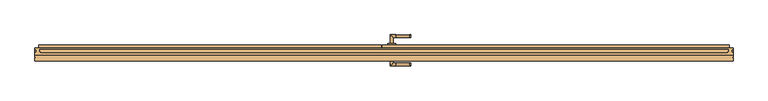
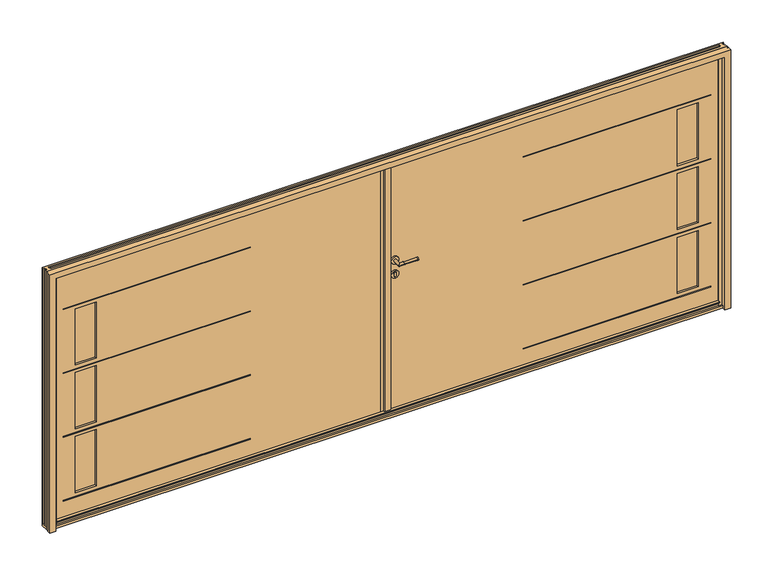
"""IFC4 building model written with IfcOpenShell, lengths in millimetres: door geometry."""

from ifc_helpers import new_model, si_unit, point, frame, frame_2d, origin, origin_with_axes, place, context, project, spatial, polyline, circle_curve, ellipse_curve, trimmed, segment, composite_curve, outline, extrude, faceted_brep, source, transform, mapped, element, save
from ifc_brep_helpers import plane_surface, cylinder_surface, advanced_brep


def door_2a186d26(model_context):
    return source(origin(), model_context, "Body", "SolidModel", [
        extrude(outline(polyline([(2198.0, 21.5), (82.0, 21.5), (82.0, 49.5), (2198.0, 49.5), (2198.0, 21.5)])), frame((0.0, 0.0, 108.0), z_axis=(0.0, 0.0, 1.0), x_axis=(1.0, 0.0, 0.0)), (0.0, 0.0, 1.0), 1633.8),
        advanced_brep(
        [(60.1308541, 82.5, 1120.0), (41.1308541, 82.5, 1120.0), (60.1308541, 123.5, 1120.0), (41.1308541, 142.5, 1120.0), (176.1308541, 123.5, 1120.0), (176.1308541, 142.5, 1120.0), (79.1308541, 123.5, 1120.0), (79.1308541, 142.5, 1120.0), (170.1308541, 142.5, 1120.0), (170.1308541, 123.5, 1120.0), (170.1308541, 124.0, 1120.0), (170.1308541, 142.0, 1120.0), (79.1308541, 124.0, 1120.0), (79.1308541, 142.0, 1120.0)],
        [
            (0, 1, circle_curve(frame((50.6308541, 82.5, 1120.0), z_axis=(0.0, -1.0, 0.0), x_axis=(-1.0, 0.0, 0.0)), 9.5)),
            (1, 0, circle_curve(frame((50.6308541, 82.5, 1120.0), z_axis=(0.0, -1.0, 0.0), x_axis=(-1.0, 0.0, 0.0)), 9.5)),
            (0, 2),
            (2, 3, ellipse_curve(frame((50.6308541, 133.0, 1120.0), z_axis=(-0.7071067811865475, -0.7071067811865475, 0.0), x_axis=(0.7071067811865474, -0.7071067811865476, 0.0)), 13.4350288, 9.5)),
            (3, 1),
            (3, 2, ellipse_curve(frame((50.6308541, 133.0, 1120.0), z_axis=(-0.7071067811865475, -0.7071067811865475, 0.0), x_axis=(0.7071067811865474, -0.7071067811865476, 0.0)), 13.4350288, 9.5)),
            (4, 5, circle_curve(frame((176.1308541, 133.0, 1120.0), z_axis=(1.0, 0.0, 0.0), x_axis=(0.0, 1.0, 0.0)), 9.5)),
            (5, 4, circle_curve(frame((176.1308541, 133.0, 1120.0), z_axis=(1.0, 0.0, 0.0), x_axis=(0.0, 1.0, 0.0)), 9.5)),
            (2, 6),
            (6, 7, circle_curve(frame((79.1308541, 133.0, 1120.0), z_axis=(-1.0, 0.0, 0.0), x_axis=(0.0, 1.0, 0.0)), 9.5)),
            (7, 3),
            (5, 8),
            (8, 9, circle_curve(frame((170.1308541, 133.0, 1120.0), z_axis=(1.0, 0.0, 0.0), x_axis=(0.0, 1.0, 0.0)), 9.5)),
            (9, 4),
            (7, 6, circle_curve(frame((79.1308541, 133.0, 1120.0), z_axis=(-1.0, 0.0, 0.0), x_axis=(0.0, 1.0, 0.0)), 9.5)),
            (9, 8, circle_curve(frame((170.1308541, 133.0, 1120.0), z_axis=(1.0, 0.0, 0.0), x_axis=(0.0, 1.0, 0.0)), 9.5)),
            (10, 11, circle_curve(frame((170.1308541, 133.0, 1120.0), z_axis=(1.0, 0.0, 0.0), x_axis=(0.0, 1.0, 0.0)), 9.0)),
            (11, 10, circle_curve(frame((170.1308541, 133.0, 1120.0), z_axis=(1.0, 0.0, 0.0), x_axis=(0.0, 1.0, 0.0)), 9.0)),
            (12, 13, circle_curve(frame((79.1308541, 133.0, 1120.0), z_axis=(-1.0, 0.0, 0.0), x_axis=(0.0, 1.0, 0.0)), 9.0)),
            (13, 12, circle_curve(frame((79.1308541, 133.0, 1120.0), z_axis=(-1.0, 0.0, 0.0), x_axis=(0.0, 1.0, 0.0)), 9.0)),
            (11, 13),
            (12, 10),
        ],
        [
            plane_surface(frame((50.6308541, 82.5, 1120.0), z_axis=(0.0, -1.0, 0.0), x_axis=(0.0, 0.0, 1.0))),
            cylinder_surface(frame((50.6308541, 82.5, 1120.0), z_axis=(0.0, -1.0, 0.0), x_axis=(-1.0, 0.0, 0.0)), 9.5),
            plane_surface(frame((176.1308541, 133.0, 1120.0), z_axis=(1.0, 0.0, 0.0), x_axis=(0.0, 0.0, 1.0))),
            cylinder_surface(frame((50.6308541, 133.0, 1120.0), z_axis=(-1.0, 0.0, 0.0), x_axis=(0.0, 1.0, 0.0)), 9.5),
            plane_surface(frame((170.1308541, 142.5, 1120.0), z_axis=(-1.0, 0.0, 0.0), x_axis=(0.0, 0.0, 1.0))),
            plane_surface(frame((79.1308541, 142.5, 1120.0), z_axis=(1.0, 0.0, 0.0), x_axis=(0.0, 0.0, -1.0))),
            cylinder_surface(frame((50.6308541, 133.0, 1120.0), z_axis=(-1.0, 0.0, 0.0), x_axis=(0.0, 1.0, 0.0)), 9.0),
        ],
        [
            (0, [[1, 2]]),
            (1, [[-1, 3, 4, 5]]),
            (1, [[-2, -5, 6, -3]]),
            (2, [[7, 8]]),
            (3, [[-4, 9, 10, 11]]),
            (3, [[-8, 12, 13, 14]]),
            (3, [[-6, -11, 15, -9]]),
            (3, [[-7, -14, 16, -12]]),
            (4, [[-13, -16], [17, 18]]),
            (5, [[-10, -15], [19, 20]]),
            (6, [[-18, 21, -19, 22]]),
            (6, [[-17, -22, -20, -21]]),
        ],
    ),
        extrude(outline(composite_curve([segment(trimmed(circle_curve(frame_2d((1019.75, 50.6308541)), 26.0), [point((1019.75, 24.6308541))], [point((1019.75, 76.6308541))], False, "CARTESIAN"), True, "CONTINUOUS"), segment(trimmed(circle_curve(frame_2d((1019.75, 50.6308541)), 26.0), [point((1019.75, 76.6308541))], [point((1019.75, 24.6308541))], False, "CARTESIAN"), True, "CONTINUOUS")], self_intersect=False)), frame((0.0, 72.5, 0.0), z_axis=(0.0, 1.0, 0.0), x_axis=(0.0, 0.0, 1.0)), (0.0, 0.0, 1.0), 10.0),
        extrude(outline(composite_curve([segment(polyline([(1021.404547, 44.8808541), (1008.0, 44.8808541)]), True, "CONTINUOUS"), segment(trimmed(circle_curve(frame_2d((1008.0, 50.6308541)), 5.75), [point((1008.0, 44.8808541))], [point((1008.0, 56.3808541))], False, "CARTESIAN"), True, "CONTINUOUS"), segment(polyline([(1008.0, 56.3808541), (1021.404547, 56.3808541)]), True, "CONTINUOUS"), segment(trimmed(circle_curve(frame_2d((1028.0, 50.6308541)), 8.75), [point((1021.404547, 56.3808541))], [point((1021.404547, 44.8808541))], False, "CARTESIAN"), True, "CONTINUOUS")], self_intersect=False)), frame((0.0, 82.5, 0.0), z_axis=(0.0, 1.0, 0.0), x_axis=(0.0, 0.0, 1.0)), (0.0, 0.0, 1.0), 1.0),
        extrude(outline(composite_curve([segment(trimmed(circle_curve(frame_2d((1120.0, 50.6308541)), 26.0), [point((1120.0, 24.6308541))], [point((1120.0, 76.6308541))], False, "CARTESIAN"), True, "CONTINUOUS"), segment(trimmed(circle_curve(frame_2d((1120.0, 50.6308541)), 26.0), [point((1120.0, 76.6308541))], [point((1120.0, 24.6308541))], False, "CARTESIAN"), True, "CONTINUOUS")], self_intersect=False)), frame((0.0, 72.5, 0.0), z_axis=(0.0, 1.0, 0.0), x_axis=(0.0, 0.0, 1.0)), (0.0, 0.0, 1.0), 10.0),
        advanced_brep(
        [(60.1308541, -4.5, 1120.0), (41.1308541, -4.5, 1120.0), (41.1308541, -64.5, 1120.0), (60.1308541, -45.5, 1120.0), (176.1308541, -45.5, 1120.0), (176.1308541, -64.5, 1120.0), (170.1308541, -45.5, 1120.0), (170.1308541, -64.5, 1120.0), (79.1308541, -64.5, 1120.0), (79.1308541, -45.5, 1120.0), (170.1308541, -46.0, 1120.0), (170.1308541, -64.0, 1120.0), (79.1308541, -46.0, 1120.0), (79.1308541, -64.0, 1120.0)],
        [
            (0, 1, circle_curve(frame((50.6308541, -4.5, 1120.0), z_axis=(0.0, 1.0, 0.0), x_axis=(-1.0, 0.0, 0.0)), 9.5)),
            (1, 0, circle_curve(frame((50.6308541, -4.5, 1120.0), z_axis=(0.0, 1.0, 0.0), x_axis=(-1.0, 0.0, 0.0)), 9.5)),
            (1, 2),
            (2, 3, ellipse_curve(frame((50.6308541, -55.0, 1120.0), z_axis=(-0.7071067811865475, 0.7071067811865475, 0.0), x_axis=(0.7071067811865474, 0.7071067811865476, 0.0)), 13.4350288, 9.5)),
            (3, 0),
            (3, 2, ellipse_curve(frame((50.6308541, -55.0, 1120.0), z_axis=(-0.7071067811865475, 0.7071067811865475, 0.0), x_axis=(0.7071067811865474, 0.7071067811865476, 0.0)), 13.4350288, 9.5)),
            (4, 5, circle_curve(frame((176.1308541, -55.0, 1120.0), z_axis=(1.0, 0.0, 0.0), x_axis=(0.0, -1.0, 0.0)), 9.5)),
            (5, 4, circle_curve(frame((176.1308541, -55.0, 1120.0), z_axis=(1.0, 0.0, 0.0), x_axis=(0.0, -1.0, 0.0)), 9.5)),
            (4, 6),
            (6, 7, circle_curve(frame((170.1308541, -55.0, 1120.0), z_axis=(1.0, 0.0, 0.0), x_axis=(0.0, -1.0, 0.0)), 9.5)),
            (7, 5),
            (2, 8),
            (8, 9, circle_curve(frame((79.1308541, -55.0, 1120.0), z_axis=(-1.0, 0.0, 0.0), x_axis=(0.0, -1.0, 0.0)), 9.5)),
            (9, 3),
            (9, 8, circle_curve(frame((79.1308541, -55.0, 1120.0), z_axis=(-1.0, 0.0, 0.0), x_axis=(0.0, -1.0, 0.0)), 9.5)),
            (7, 6, circle_curve(frame((170.1308541, -55.0, 1120.0), z_axis=(1.0, 0.0, 0.0), x_axis=(0.0, -1.0, 0.0)), 9.5)),
            (10, 11, circle_curve(frame((170.1308541, -55.0, 1120.0), z_axis=(1.0, 0.0, 0.0), x_axis=(0.0, -1.0, 0.0)), 9.0)),
            (11, 10, circle_curve(frame((170.1308541, -55.0, 1120.0), z_axis=(1.0, 0.0, 0.0), x_axis=(0.0, -1.0, 0.0)), 9.0)),
            (12, 13, circle_curve(frame((79.1308541, -55.0, 1120.0), z_axis=(-1.0, 0.0, 0.0), x_axis=(0.0, -1.0, 0.0)), 9.0)),
            (13, 12, circle_curve(frame((79.1308541, -55.0, 1120.0), z_axis=(-1.0, 0.0, 0.0), x_axis=(0.0, -1.0, 0.0)), 9.0)),
            (10, 12),
            (13, 11),
        ],
        [
            plane_surface(frame((50.6308541, -4.5, 1120.0), z_axis=(0.0, 1.0, 0.0), x_axis=(0.0, 0.0, 1.0))),
            cylinder_surface(frame((50.6308541, -4.5, 1120.0), z_axis=(0.0, 1.0, 0.0), x_axis=(-1.0, 0.0, 0.0)), 9.5),
            plane_surface(frame((176.1308541, -55.0, 1120.0), z_axis=(1.0, 0.0, 0.0), x_axis=(0.0, 0.0, 1.0))),
            cylinder_surface(frame((50.6308541, -55.0, 1120.0), z_axis=(-1.0, 0.0, 0.0), x_axis=(0.0, -1.0, 0.0)), 9.5),
            plane_surface(frame((170.1308541, -64.5, 1120.0), z_axis=(-1.0, 0.0, 0.0), x_axis=(0.0, 0.0, 1.0))),
            plane_surface(frame((79.1308541, -64.5, 1120.0), z_axis=(1.0, 0.0, 0.0), x_axis=(0.0, 0.0, -1.0))),
            cylinder_surface(frame((50.6308541, -55.0, 1120.0), z_axis=(-1.0, 0.0, 0.0), x_axis=(0.0, -1.0, 0.0)), 9.0),
        ],
        [
            (0, [[1, 2]]),
            (1, [[3, 4, 5, -2]]),
            (1, [[-5, 6, -3, -1]]),
            (2, [[7, 8]]),
            (3, [[9, 10, 11, -7]]),
            (3, [[12, 13, 14, -4]]),
            (3, [[-14, 15, -12, -6]]),
            (3, [[-11, 16, -9, -8]]),
            (4, [[-16, -10], [17, 18]]),
            (5, [[-15, -13], [19, 20]]),
            (6, [[21, -20, 22, -17]]),
            (6, [[-22, -19, -21, -18]]),
        ],
    ),
        extrude(outline(composite_curve([segment(trimmed(circle_curve(frame_2d((1019.75, 50.6308541)), 26.0), [point((1019.75, 24.6308541))], [point((1019.75, 76.6308541))], False, "CARTESIAN"), True, "CONTINUOUS"), segment(trimmed(circle_curve(frame_2d((1019.75, 50.6308541)), 26.0), [point((1019.75, 76.6308541))], [point((1019.75, 24.6308541))], False, "CARTESIAN"), True, "CONTINUOUS")], self_intersect=False)), frame((0.0, -4.5, 0.0), z_axis=(0.0, 1.0, 0.0), x_axis=(0.0, 0.0, 1.0)), (0.0, 0.0, 1.0), 10.0),
        extrude(outline(composite_curve([segment(polyline([(1021.404547, 44.8808541), (1008.0, 44.8808541)]), True, "CONTINUOUS"), segment(trimmed(circle_curve(frame_2d((1008.0, 50.6308541)), 5.75), [point((1008.0, 44.8808541))], [point((1008.0, 56.3808541))], False, "CARTESIAN"), True, "CONTINUOUS"), segment(polyline([(1008.0, 56.3808541), (1021.404547, 56.3808541)]), True, "CONTINUOUS"), segment(trimmed(circle_curve(frame_2d((1028.0, 50.6308541)), 8.75), [point((1021.404547, 56.3808541))], [point((1021.404547, 44.8808541))], False, "CARTESIAN"), True, "CONTINUOUS")], self_intersect=False)), frame((0.0, -5.5, 0.0), z_axis=(0.0, 1.0, 0.0), x_axis=(0.0, 0.0, 1.0)), (0.0, 0.0, 1.0), 1.0),
        extrude(outline(composite_curve([segment(trimmed(circle_curve(frame_2d((1120.0, 50.6308541)), 26.0), [point((1120.0, 24.6308541))], [point((1120.0, 76.6308541))], False, "CARTESIAN"), True, "CONTINUOUS"), segment(trimmed(circle_curve(frame_2d((1120.0, 50.6308541)), 26.0), [point((1120.0, 76.6308541))], [point((1120.0, 24.6308541))], False, "CARTESIAN"), True, "CONTINUOUS")], self_intersect=False)), frame((0.0, -4.5, 0.0), z_axis=(0.0, 1.0, 0.0), x_axis=(0.0, 0.0, 1.0)), (0.0, 0.0, 1.0), 10.0),
        faceted_brep([(2262.0, 5.5, 1805.8), (2262.0, 5.5, 44.0), (2262.0, 21.4981764, 44.0), (2262.0, 21.4981764, 1805.8), (18.0, 21.5, 44.0), (18.0, 21.5, 1805.8), (1979.0, 21.5, 659.6), (2123.0, 21.5, 659.6), (2123.0, 21.5, 1065.7), (1979.0, 21.5, 1065.7), (1979.0, 21.5, 199.0), (2123.0, 21.5, 199.0), (2123.0, 21.5, 605.1), (1979.0, 21.5, 605.1), (1979.0, 21.5, 1120.2), (2123.0, 21.5, 1120.2), (2123.0, 21.5, 1526.3), (1979.0, 21.5, 1526.3), (18.0, 5.5, 44.0), (18.0, 5.5, 1805.8), (1979.0, 5.5, 1065.7), (1979.0, 5.5, 659.6), (2123.0, 5.5, 1065.7), (2123.0, 5.5, 659.6), (1979.0, 5.5, 605.1), (1979.0, 5.5, 199.0), (2123.0, 5.5, 605.1), (2123.0, 5.5, 199.0), (930.0, 5.5, 1094.2), (2206.0, 5.5, 1094.2), (2206.0, 5.5, 1089.2), (930.0, 5.5, 1089.2), (930.0, 5.5, 633.6), (2206.0, 5.5, 633.6), (2206.0, 5.5, 628.6), (930.0, 5.5, 628.6), (930.0, 5.5, 173.0), (2206.0, 5.5, 173.0), (2206.0, 5.5, 168.0), (930.0, 5.5, 168.0), (1979.0, 5.5, 1526.3), (2123.0, 5.5, 1526.3), (2123.0, 5.5, 1120.2), (1979.0, 5.5, 1120.2), (930.0, 5.5, 1554.8), (2206.0, 5.5, 1554.8), (2206.0, 5.5, 1549.8), (930.0, 5.5, 1549.8), (930.0, 14.5185028, 1094.2), (930.0, 14.5185028, 1089.2), (2206.0, 14.5185028, 1089.2), (2206.0, 14.5185028, 1094.2), (930.0, 14.5185028, 633.6), (930.0, 14.5185028, 628.6), (2206.0, 14.5185028, 628.6), (2206.0, 14.5185028, 633.6), (930.0, 14.5185028, 173.0), (930.0, 14.5185028, 168.0), (2206.0, 14.5185028, 168.0), (2206.0, 14.5185028, 173.0), (930.0, 14.5185028, 1554.8), (930.0, 14.5185028, 1549.8), (2206.0, 14.5185028, 1549.8), (2206.0, 14.5185028, 1554.8)], [[[0, 1, 2, 3]], [[2, 4, 5, 3], [6, 7, 8, 9], [10, 11, 12, 13], [14, 15, 16, 17]], [[18, 19, 5, 4]], [[1, 18, 4, 2]], [[6, 9, 20, 21]], [[9, 8, 22, 20]], [[23, 22, 8, 7]], [[21, 23, 7, 6]], [[10, 13, 24, 25]], [[13, 12, 26, 24]], [[27, 26, 12, 11]], [[25, 27, 11, 10]], [[0, 19, 18, 1], [20, 22, 23, 21], [24, 26, 27, 25], [28, 29, 30, 31], [32, 33, 34, 35], [36, 37, 38, 39], [40, 41, 42, 43], [44, 45, 46, 47]], [[48, 28, 31, 49]], [[49, 31, 30, 50]], [[50, 30, 29, 51]], [[52, 32, 35, 53]], [[53, 35, 34, 54]], [[54, 34, 33, 55]], [[55, 33, 32, 52]], [[56, 36, 39, 57]], [[57, 39, 38, 58]], [[58, 38, 37, 59]], [[59, 37, 36, 56]], [[52, 53, 54, 55]], [[57, 58, 59, 56]], [[60, 61, 62, 63]], [[48, 49, 50, 51]], [[3, 5, 19, 0]], [[14, 17, 40, 43]], [[43, 42, 15, 14]], [[42, 41, 16, 15]], [[17, 16, 41, 40]], [[60, 44, 47, 61]], [[61, 47, 46, 62]], [[62, 46, 45, 63]], [[63, 45, 44, 60]], [[51, 29, 28, 48]]]),
        faceted_brep([(2292.0, 53.5, 1835.8), (2292.0, 53.5, 14.0), (2292.0, 72.5, 14.0), (2292.0, 72.5, 1835.8), (-12.0, 72.5, 14.0), (-12.0, 72.5, 1835.8), (930.0, 72.5, 1089.2), (2206.0, 72.5, 1089.2), (2206.0, 72.5, 1094.2), (930.0, 72.5, 1094.2), (1979.0, 72.5, 1065.7), (1979.0, 72.5, 659.6), (2123.0, 72.5, 659.6), (2123.0, 72.5, 1065.7), (1979.0, 72.5, 605.1), (1979.0, 72.5, 199.0), (2123.0, 72.5, 199.0), (2123.0, 72.5, 605.1), (930.0, 72.5, 628.6), (2206.0, 72.5, 628.6), (2206.0, 72.5, 633.6), (930.0, 72.5, 633.6), (930.0, 72.5, 168.0), (2206.0, 72.5, 168.0), (2206.0, 72.5, 173.0), (930.0, 72.5, 173.0), (1979.0, 72.5, 1526.3), (1979.0, 72.5, 1120.2), (2123.0, 72.5, 1120.2), (2123.0, 72.5, 1526.3), (930.0, 72.5, 1549.8), (2206.0, 72.5, 1549.8), (2206.0, 72.5, 1554.8), (930.0, 72.5, 1554.8), (-12.0, 53.5, 14.0), (-12.0, 53.5, 1835.8), (2123.0, 49.5, 1065.7), (1979.0, 49.5, 1065.7), (2123.0, 49.4981764, 659.6), (1979.0, 49.5, 659.6), (2123.0, 49.5, 605.1), (1979.0, 49.5, 605.1), (2123.0, 49.4981764, 199.0), (1979.0, 49.5, 199.0), (930.0, 63.0, 1089.2), (930.0, 63.0, 1094.2), (2206.0, 63.0, 1094.2), (2206.0, 63.0, 1089.2), (930.0, 63.0, 628.6), (930.0, 63.0, 633.6), (2206.0, 63.0, 633.6), (2206.0, 63.0, 628.6), (930.0, 63.0, 168.0), (930.0, 63.0, 173.0), (2206.0, 63.0, 173.0), (2206.0, 63.0, 168.0), (2198.0, 49.5, 1741.8), (82.0, 49.5, 1741.8), (82.0, 49.5, 108.0), (2198.0, 49.5, 108.0), (2123.0, 49.5, 1526.3), (2123.0, 49.5, 1120.2), (1979.0, 49.5, 1120.2), (1979.0, 49.5, 1526.3), (2198.0, 21.5, 108.0), (2198.0, 21.5, 1741.8), (82.0, 21.5, 108.0), (82.0, 21.5, 1741.8), (2262.0, 53.5, 44.0), (18.0, 53.5, 44.0), (18.0, 53.5, 1805.8), (2262.0, 53.5, 1805.8), (2262.0, 21.5, 1805.8), (2262.0, 21.5, 44.0), (18.0, 21.5, 44.0), (18.0, 21.5, 1805.8), (930.0, 63.0, 1554.8), (2206.0, 63.0, 1554.8), (2206.0, 63.0, 1549.8), (930.0, 63.0, 1549.8)], [[[0, 1, 2, 3]], [[2, 4, 5, 3], [6, 7, 8, 9], [10, 11, 12, 13], [14, 15, 16, 17], [18, 19, 20, 21], [22, 23, 24, 25], [26, 27, 28, 29], [30, 31, 32, 33]], [[34, 35, 5, 4]], [[1, 34, 4, 2]], [[36, 37, 10, 13]], [[13, 12, 38, 36]], [[39, 38, 12, 11]], [[37, 39, 11, 10]], [[40, 41, 14, 17]], [[17, 16, 42, 40]], [[43, 42, 16, 15]], [[41, 43, 15, 14]], [[44, 6, 9, 45]], [[46, 8, 7, 47]], [[47, 7, 6, 44]], [[48, 18, 21, 49]], [[49, 21, 20, 50]], [[50, 20, 19, 51]], [[51, 19, 18, 48]], [[52, 22, 25, 53]], [[53, 25, 24, 54]], [[54, 24, 23, 55]], [[55, 23, 22, 52]], [[56, 57, 58, 59], [36, 38, 39, 37], [40, 42, 43, 41], [60, 61, 62, 63]], [[56, 59, 64, 65]], [[59, 58, 66, 64]], [[58, 57, 67, 66]], [[0, 35, 34, 1], [68, 69, 70, 71]], [[72, 73, 68, 71]], [[73, 74, 69, 68]], [[72, 75, 74, 73], [64, 66, 67, 65]], [[74, 75, 70, 69]], [[45, 46, 47, 44]], [[49, 50, 51, 48]], [[53, 54, 55, 52]], [[76, 77, 78, 79]], [[3, 5, 35, 0]], [[71, 70, 75, 72]], [[65, 67, 57, 56]], [[60, 63, 26, 29]], [[63, 62, 27, 26]], [[62, 61, 28, 27]], [[29, 28, 61, 60]], [[79, 30, 33, 76]], [[78, 31, 30, 79]], [[77, 32, 31, 78]], [[76, 33, 32, 77]], [[45, 9, 8, 46]]]),
        extrude(outline(polyline([(-2198.0, 21.5), (-2198.0, 49.5), (-41.0, 49.5), (-41.0, 21.5), (-2198.0, 21.5)])), frame((0.0, 0.0, 108.0), z_axis=(0.0, 0.0, 1.0), x_axis=(1.0, 0.0, 0.0)), (0.0, 0.0, 1.0), 1633.8),
        faceted_brep([(-17.0, 53.5, 44.0), (-17.0, 53.5, 14.0), (-17.0, 72.5, 14.0), (-17.0, 72.5, 1835.8), (-17.0, 53.5, 1835.8), (-17.0, 53.5, 1805.8), (-2262.0, 53.5, 44.0), (-2262.0, 53.5, 1805.8), (-2292.0, 53.5, 1835.8), (-2292.0, 53.5, 14.0), (-2292.0, 72.5, 14.0), (-2292.0, 72.5, 1835.8), (-1979.0, 72.5, 1065.7), (-2123.0, 72.5, 1065.7), (-2123.0, 72.5, 659.6), (-1979.0, 72.5, 659.6), (-1979.0, 72.5, 605.1), (-2123.0, 72.5, 605.1), (-2123.0, 72.5, 199.0), (-1979.0, 72.5, 199.0), (-2206.0, 72.5, 628.6), (-930.0, 72.5, 628.6), (-930.0, 72.5, 633.6), (-2206.0, 72.5, 633.6), (-2206.0, 72.5, 168.0), (-930.0, 72.5, 168.0), (-930.0, 72.5, 173.0), (-2206.0, 72.5, 173.0), (-1979.0, 72.5, 1526.3), (-2123.0, 72.5, 1526.3), (-2123.0, 72.5, 1120.2), (-1979.0, 72.5, 1120.2), (-2206.0, 72.5, 1549.8), (-930.0, 72.5, 1549.8), (-930.0, 72.5, 1554.8), (-2206.0, 72.5, 1554.8), (-2206.0, 72.5, 1089.2), (-930.0, 72.5, 1089.2), (-930.0, 72.5, 1094.2), (-2206.0, 72.5, 1094.2), (-6.0, 53.5, 1805.8), (-6.0, 53.5, 44.0), (-2123.0, 49.5, 1065.7), (-2123.0, 49.4981764, 659.6), (-1979.0, 49.5, 659.6), (-1979.0, 49.5, 1065.7), (-1979.0, 49.5, 605.1), (-2123.0, 49.4981764, 605.1), (-2123.0, 49.4981764, 199.0), (-1979.0, 49.5, 199.0), (-2206.0, 67.5, 628.6), (-930.0, 67.5, 628.6), (-930.0, 67.5, 633.6), (-2206.0, 67.5, 633.6), (-2206.0, 67.5, 168.0), (-930.0, 67.5, 168.0), (-930.0, 67.5, 173.0), (-2206.0, 67.5, 173.0), (-2198.0, 49.4981764, 108.0), (-2198.0, 49.4981764, 1741.8), (-2198.0, 21.4981764, 1741.8), (-2198.0, 21.4981764, 108.0), (-41.0, 49.4981764, 108.0), (-41.0, 49.4981764, 1741.8), (-2123.0, 49.4981764, 1526.3), (-1979.0, 49.4981764, 1526.3), (-1979.0, 49.4981764, 1120.2), (-2123.0, 49.4981764, 1120.2), (-41.0, 21.4981764, 108.0), (-41.0, 21.4981764, 1741.8), (-2262.0, 21.4981764, 1805.8), (-2262.0, 21.4981764, 44.0), (-6.0, 21.4981764, 44.0), (-6.0, 21.4981764, 1805.8), (-930.0, 67.5, 1549.8), (-2206.0, 67.5, 1549.8), (-2206.0, 67.5, 1554.8), (-930.0, 67.5, 1554.8), (-930.0, 67.5, 1089.2), (-2206.0, 67.5, 1089.2), (-2206.0, 67.5, 1094.2), (-930.0, 67.5, 1094.2)], [[[0, 1, 2, 3, 4, 5]], [[1, 0, 6, 7, 5, 4, 8, 9]], [[2, 1, 9, 10]], [[2, 10, 11, 3], [12, 13, 14, 15], [16, 17, 18, 19], [20, 21, 22, 23], [24, 25, 26, 27], [28, 29, 30, 31], [32, 33, 34, 35], [36, 37, 38, 39]], [[5, 40, 41, 0]], [[11, 10, 9, 8]], [[13, 42, 43, 14]], [[44, 15, 14, 43]], [[45, 12, 15, 44]], [[16, 46, 47, 17]], [[17, 47, 48, 18]], [[49, 19, 18, 48]], [[46, 16, 19, 49]], [[50, 51, 21, 20]], [[51, 52, 22, 21]], [[52, 53, 23, 22]], [[53, 50, 20, 23]], [[54, 55, 25, 24]], [[55, 56, 26, 25]], [[56, 57, 27, 26]], [[57, 54, 24, 27]], [[58, 59, 60, 61]], [[59, 58, 62, 63], [42, 45, 44, 43], [47, 46, 49, 48], [64, 65, 66, 67]], [[58, 61, 68, 62]], [[68, 69, 63, 62]], [[70, 71, 72, 73], [61, 60, 69, 68]], [[71, 70, 7, 6]], [[71, 6, 0, 41, 72]], [[40, 73, 72, 41]], [[51, 50, 53, 52]], [[55, 54, 57, 56]], [[74, 75, 76, 77]], [[78, 79, 80, 81]], [[60, 59, 63, 69]], [[3, 11, 8, 4]], [[7, 70, 73, 40, 5]], [[28, 65, 64, 29]], [[65, 28, 31, 66]], [[66, 31, 30, 67]], [[29, 64, 67, 30]], [[12, 45, 42, 13]], [[75, 74, 33, 32]], [[76, 75, 32, 35]], [[77, 76, 35, 34]], [[74, 77, 34, 33]], [[79, 78, 37, 36]], [[80, 79, 36, 39]], [[81, 80, 39, 38]], [[78, 81, 38, 37]]]),
        extrude(outline(polyline([(18.0, 5.5), (-41.0, 5.5), (-41.0, 21.5), (18.0, 21.5), (18.0, 5.5)])), frame((0.0, 0.0, 44.0), z_axis=(0.0, 0.0, 1.0), x_axis=(1.0, 0.0, 0.0)), (0.0, 0.0, 1.0), 1761.8),
        faceted_brep([(23.5, 5.5, 49.0), (21.5, -2.5, 49.0), (-20.5, -2.5, 49.0), (-22.5, 5.5, 49.0), (23.5, 5.5, 1801.3), (21.5, -2.5, 1801.3), (-20.5, -2.5, 1801.3), (-22.5, 5.5, 1801.3)], [[[0, 1, 2, 3]], [[4, 5, 1, 0]], [[5, 6, 2, 1]], [[6, 7, 3, 2]], [[7, 4, 0, 3]], [[4, 7, 6, 5]]]),
        faceted_brep([(-41.0, 5.5, 44.0), (-41.0, 21.4981764, 44.0), (-41.0, 21.4981764, 1805.8), (-41.0, 5.5, 1805.8), (-2262.0, 5.5, 44.0), (-2262.0, 21.4981764, 44.0), (-2262.0, 21.4981764, 1805.8), (-1979.0, 21.4981764, 1065.7), (-2123.0, 21.4981764, 1065.7), (-2123.0, 21.4981764, 659.6), (-1979.0, 21.4981764, 659.6), (-1979.0, 21.4981764, 605.1), (-2123.0, 21.4981764, 605.1), (-2123.0, 21.4981764, 199.0), (-1979.0, 21.4981764, 199.0), (-1979.0, 21.4981764, 1526.3), (-2123.0, 21.4981764, 1526.3), (-2123.0, 21.4981764, 1120.2), (-1979.0, 21.4981764, 1120.2), (-2262.0, 5.5, 1805.8), (-2123.0, 5.5, 1065.7), (-1979.0, 5.5, 1065.7), (-1979.0, 5.5, 659.6), (-2123.0, 5.5, 659.6), (-2123.0, 5.5, 605.1), (-1979.0, 5.5, 605.1), (-1979.0, 5.5, 199.0), (-2123.0, 5.5, 199.0), (-2206.0, 5.5, 633.6), (-930.0, 5.5, 633.6), (-930.0, 5.5, 628.6), (-2206.0, 5.5, 628.6), (-2206.0, 5.5, 173.0), (-930.0, 5.5, 173.0), (-930.0, 5.5, 168.0), (-2206.0, 5.5, 168.0), (-2123.0, 5.5, 1526.3), (-1979.0, 5.5, 1526.3), (-1979.0, 5.5, 1120.2), (-2123.0, 5.5, 1120.2), (-2206.0, 5.5, 1094.2), (-930.0, 5.5, 1094.2), (-930.0, 5.5, 1089.2), (-2206.0, 5.5, 1089.2), (-2206.0, 5.5, 1549.8), (-2206.0, 5.5, 1554.8), (-930.0, 5.5, 1554.8), (-930.0, 5.5, 1549.8), (-2206.0, 10.5, 633.6), (-930.0, 10.5, 633.6), (-930.0, 10.5, 628.6), (-2206.0, 10.5, 628.6), (-2206.0, 10.5, 173.0), (-930.0, 10.5, 173.0), (-930.0, 10.5, 168.0), (-2206.0, 10.5, 168.0), (-2206.0, 10.5, 1094.2), (-2206.0, 10.5, 1089.2), (-930.0, 10.5, 1089.2), (-930.0, 10.5, 1094.2), (-2206.0, 10.5, 1549.8), (-930.0, 10.5, 1549.8), (-930.0, 10.5, 1554.8), (-2206.0, 10.5, 1554.8)], [[[0, 1, 2, 3]], [[1, 0, 4, 5]], [[1, 5, 6, 2], [7, 8, 9, 10], [11, 12, 13, 14], [15, 16, 17, 18]], [[3, 19, 4, 0], [20, 21, 22, 23], [24, 25, 26, 27], [28, 29, 30, 31], [32, 33, 34, 35], [36, 37, 38, 39], [40, 41, 42, 43], [44, 45, 46, 47]], [[4, 19, 6, 5]], [[11, 25, 24, 12]], [[25, 11, 14, 26]], [[26, 14, 13, 27]], [[12, 24, 27, 13]], [[21, 7, 10, 22]], [[22, 10, 9, 23]], [[8, 20, 23, 9]], [[48, 49, 29, 28]], [[49, 50, 30, 29]], [[50, 51, 31, 30]], [[51, 48, 28, 31]], [[52, 53, 33, 32]], [[53, 54, 34, 33]], [[54, 55, 35, 34]], [[55, 52, 32, 35]], [[48, 51, 50, 49]], [[52, 55, 54, 53]], [[56, 57, 58, 59]], [[60, 61, 62, 63]], [[3, 2, 6, 19]], [[7, 21, 20, 8]], [[15, 37, 36, 16]], [[37, 15, 18, 38]], [[38, 18, 17, 39]], [[16, 36, 39, 17]], [[56, 59, 41, 40]], [[59, 58, 42, 41]], [[58, 57, 43, 42]], [[57, 56, 40, 43]], [[60, 63, 45, 44]], [[63, 62, 46, 45]], [[62, 61, 47, 46]], [[61, 60, 44, 47]]]),
        faceted_brep([(2280.0, -33.9665116, 0.0), (2280.0, -2.5, 0.0), (2257.5, -2.5, 0.0), (2257.5, 5.5, 0.0), (2319.0, 5.5, 0.0), (2319.0, -6.5, 0.0), (2314.0, -6.5, 0.0), (2314.0, -11.5, 0.0), (2319.0, -11.5, 0.0), (2319.0, -33.9665116, 0.0), (-2319.0, -6.5, 0.0), (-2319.0, 5.5, 0.0), (-2257.5, 5.5, 0.0), (-2257.5, -2.5, 0.0), (-2280.0, -2.5, 0.0), (-2280.0, -33.9665116, 0.0), (-2319.0, -33.9665116, 0.0), (-2319.0, -11.5, 0.0), (-2314.0, -11.5, 0.0), (-2314.0, -6.5, 0.0), (2280.0, -33.9665116, 1823.8), (2280.0, -2.5, 1823.8), (2257.5, -2.5, 1801.3), (2257.5, 5.5, 1801.3), (-2280.0, -33.9665116, 1823.8), (-2280.0, -2.5, 1823.8), (-2257.5, -2.5, 1801.3), (-2257.5, 5.5, 1801.3), (-2319.0, 5.5, 1862.8), (-2319.0, -6.5, 1862.8), (-2319.0, -11.5, 1862.8), (-2319.0, -33.9665116, 1862.8), (-2314.0, -11.5, 1862.8), (-2314.0, -6.5, 1862.8), (2319.0, -6.5, 1862.8), (2319.0, 5.5, 1862.8), (2314.0, -6.5, 1862.8), (2314.0, -11.5, 1862.8), (2319.0, -11.5, 1862.8), (2319.0, -33.9665116, 1862.8)], [[[0, 1, 2, 3, 4, 5, 6, 7, 8, 9]], [[10, 11, 12, 13, 14, 15, 16, 17, 18, 19]], [[0, 20, 21, 1]], [[2, 22, 23, 3]], [[24, 25, 21, 20]], [[26, 27, 23, 22]], [[12, 27, 26, 13]], [[25, 24, 15, 14]], [[28, 11, 10, 29]], [[30, 17, 16, 31]], [[32, 18, 17, 30]], [[33, 19, 18, 32]], [[29, 10, 19, 33]], [[34, 5, 4, 35]], [[36, 6, 5, 34]], [[37, 7, 6, 36]], [[38, 8, 7, 37]], [[39, 9, 8, 38]], [[39, 31, 16, 15, 24, 20, 0, 9]], [[1, 21, 25, 14, 13, 26, 22, 2]], [[27, 12, 11, 28, 35, 4, 3, 23]], [[39, 38, 37, 36, 34, 35, 28, 29, 33, 32, 30, 31]]]),
        faceted_brep([(2286.0, 53.5, 20.0), (2319.0, 53.5, 20.0), (2319.0, 43.5, 20.0), (2309.0, 43.5, 20.0), (2309.0, 22.5, 20.0), (2319.0, 22.5, 20.0), (2319.0, 5.5, 20.0), (2280.0, 5.5, 20.0), (2280.0, 31.5, 20.0), (2286.0, 31.5, 20.0), (-2286.0, 53.5, 20.0), (-2286.0, 31.5, 20.0), (-2280.0, 31.5, 20.0), (-2280.0, 5.5, 20.0), (-2319.0, 5.5, 20.0), (-2319.0, 22.5, 20.0), (-2309.0, 22.5, 20.0), (-2309.0, 43.5, 20.0), (-2319.0, 43.5, 20.0), (-2319.0, 53.5, 20.0), (2319.0, 53.5, 1862.8), (2286.0, 53.5, 1829.8), (-2286.0, 53.5, 1829.8), (-2319.0, 53.5, 1862.8), (2319.0, 43.5, 1862.8), (2309.0, 43.5, 1862.8), (2309.0, 22.5, 1862.8), (2319.0, 5.5, 1862.8), (-2319.0, 5.5, 1862.8), (-2280.0, 5.5, 1829.8), (2280.0, 5.5, 1829.8), (2280.0, 31.5, 1829.8), (2280.0, 31.5, 1862.8), (2280.0, 31.5, 1852.8), (2280.0, 22.5, 1852.8), (2280.0, 22.5, 1862.8), (2286.0, 31.5, 1829.8), (2286.0, 31.5, 1862.8), (2286.0, 31.5, 1852.8), (2286.0, 43.5, 1862.8), (2286.0, 43.5, 1852.8), (-2286.0, 31.5, 1829.8), (-2286.0, 31.5, 1862.8), (-2286.0, 31.5, 1852.8), (-2286.0, 43.5, 1852.8), (-2286.0, 43.5, 1862.8), (-2280.0, 31.5, 1829.8), (-2280.0, 31.5, 1862.8), (-2280.0, 31.5, 1852.8), (-2280.0, 22.5, 1862.8), (-2280.0, 22.5, 1852.8), (-2319.0, 22.5, 1862.8), (-2319.0, 43.5, 1862.8), (-2309.0, 43.5, 1862.8), (-2309.0, 22.5, 1862.8), (2319.0, 22.5, 1862.8)], [[[0, 1, 2, 3, 4, 5, 6, 7, 8, 9]], [[10, 11, 12, 13, 14, 15, 16, 17, 18, 19]], [[20, 1, 0, 21, 22, 10, 19, 23]], [[24, 2, 1, 20]], [[25, 3, 2, 24]], [[26, 4, 3, 25]], [[6, 27, 28, 14, 13, 29, 30, 7]], [[7, 30, 31, 8]], [[32, 33, 34, 35]], [[8, 31, 36, 9]], [[37, 38, 33, 32]], [[9, 36, 21, 0]], [[39, 40, 38, 37]], [[10, 22, 41, 11]], [[42, 43, 44, 45]], [[11, 41, 46, 12]], [[47, 48, 43, 42]], [[12, 46, 29, 13]], [[49, 50, 48, 47]], [[51, 15, 14, 28]], [[45, 44, 40, 39]], [[44, 43, 48, 50, 34, 33, 38, 40]], [[35, 34, 50, 49]], [[21, 36, 31, 30, 29, 46, 41, 22]], [[20, 23, 52, 53, 54, 51, 28, 27, 55, 26, 25, 24], [37, 32, 35, 49, 47, 42, 45, 39]], [[27, 6, 5, 55]], [[23, 19, 18, 52]], [[55, 5, 4, 26]], [[54, 16, 15, 51]], [[53, 17, 16, 54]], [[52, 18, 17, 53]]]),
        extrude(outline(polyline([(2.9223795, 35.1), (1.95, 32.9), (1.95, 20.0), (0.54, 20.0), (0.54, 32.9), (-0.4323795, 35.1), (2.9223795, 35.1)])), frame((-2257.5, 0.0, 0.0), z_axis=(1.0, 0.0, 0.0), x_axis=(0.0, 1.0, 0.0)), (0.0, 0.0, 1.0), 4515.0),
        extrude(outline(polyline([(-2280.0, 5.5), (2280.0, 5.5), (2280.0, -11.5), (-2280.0, -11.5), (-2280.0, 5.5)])), origin_with_axes(), (0.0, 0.0, 1.0), 20.0),
        extrude(outline(polyline([(-2319.0, 53.5), (2319.0, 53.5), (2319.0, 5.5), (-2319.0, 5.5), (-2319.0, 53.5)])), origin_with_axes(), (0.0, 0.0, 1.0), 20.0),
        extrude(outline(polyline([(5.5, 54.3693722), (5.5, 35.1), (-2.9, 35.1), (-2.9, 40.3), (3.9, 40.3), (3.9, 52.4658167), (-11.01, 49.84), (-11.01, 47.11), (-12.61, 47.11), (-12.61, 51.18), (5.5, 54.3693722)])), frame((-2257.5, 0.0, 0.0), z_axis=(1.0, 0.0, 0.0), x_axis=(0.0, 1.0, 0.0)), (0.0, 0.0, 1.0), 4515.0),
    ])


if __name__ == "__main__":
    model = new_model("IFC4")
    model_context = context("Model", 3, world=origin())
    ifc_project = project(units=[si_unit("LENGTHUNIT", "METRE", prefix="MILLI")], contexts=[model_context])
    site = spatial("IfcSite", under=ifc_project)
    building = spatial("IfcBuilding", under=site)
    placement = place(None, origin())
    door_shape = door_2a186d26(model_context)
    element("IfcDoor", 1, at=placement, inside=building, context=model_context, shape_type="MappedRepresentation", body=[
        mapped(door_shape, transform((0.0, 0.0, 0.0), x_axis=(1.0, 0.0, 0.0), y_axis=(0.0, 1.0, 0.0), z_axis=(0.0, 0.0, 1.0))),
    ])
    save(model, "model.ifc")

# Revit data of these elements
# Type
#   Type Mark = "8"
#   Version Revit = "Revit 2017"
#   Uniformat II description = "Double door"
#   Uniformat CSI = "B2030"
#   URL = "https://www.fenetremeo.com/porte-entree"
#   Type de pose = "Tunnel"
#   Référence modèle = "MeO-PE-BALADE-2vtx"
#   Pose vitrage = "Vitrage collé"
#   Keynote = "MeO-PE-BALADE-2vtx"
#   Neuf / Réno = "Rénovation"
#   Model = "Porte double BALADE"
#   Matériaux = "Aluminium / bois"
#   IFC version = "IFC 2x3 Coordination 2.0"
#   IFC classification = "Door"
#   Fiches produits = "https://www.fenetremeo.com/porte-entree"
#   Famille de produit = "Porte"
#   Manufacturer = "MéO"
#   FILE_NAME = "2021-07-MeO-PE-BALADE-2vtx"
#   Design = "Modélisation non contractuelle"
#   Description = "Porte 2 vantaux égaux"
#   Contraintes largeur porte = "700 < Largeur < 1200"
#   Contraintes hauteur porte = "1953 < Hauteur < 2500"
#   Contraintes hauteur poignée porte = "900 <Hauteur poignée < 1300"
#   Analytic Construction = "<Aucun>"
#   Coefficient thermique Ud = "0.72 / 0.75 Ud"
#   BIMobject main category = "Exterior carpentry"
#   Avis technique = "https://www.fcba.fr/wp-content/uploads/2020/10/rc_nf297.pdf"
#   Surface = 27432' - 0"
#   Pose tunnel = 0' - 0.3937"
#   Longueur de traverse haute 33,43,53,63,73,83 = 0' - 1.29921"
#   Largeur zone 2 = 3' - 3.37008"
#   Largeur zone 1 = 3' - 3.37008"
#   Largeur du dormant 33,43,53,63,73,83 = 0' - 1.29921"
#   Rough Width = 15' - 2.59843"
#   Hauteur poignée = 3' - 7.30709"
#   Hauteur dormant = 6' - 1.33858"
#   Rough Height = 6' - 1.33858"
#   HT ouvrant = 5' - 11.25197"
#   Height = 6' - 0"
#   Width = 15' - 0"
#   Doublage 75,105,125,145,165,185,205 = 0' - 3.44356"
#   Message Hors abaques = yes
#   Hors abaques = yes
#   Vitrage = Verre
#   Couleur poignée = Acier inoxydable AISI 304
#   Choix du modèle = element 399147
#   Function = (empty or 0)
#   Wall Closure = (empty or 0)
# Element 1 (IfcDoor)
#   Materials on its faces: "Acier inoxydable AISI 304", "Verre", "Aluminium"
# Materials
#   "Verre": class "Verre", colour RGB 92 99 177, transparency 0.7, Description = "Verre sodocalcique", Cost = 0
#   "Acier inoxydable AISI 304": colour RGB 120 120 120, transparency 0, Description = "Stainless Steel 18/8", Cost = 0
#   "Aluminium": colour RGB 247 247 247, transparency 0, Description = "Aluminium 6061", Cost = 0
